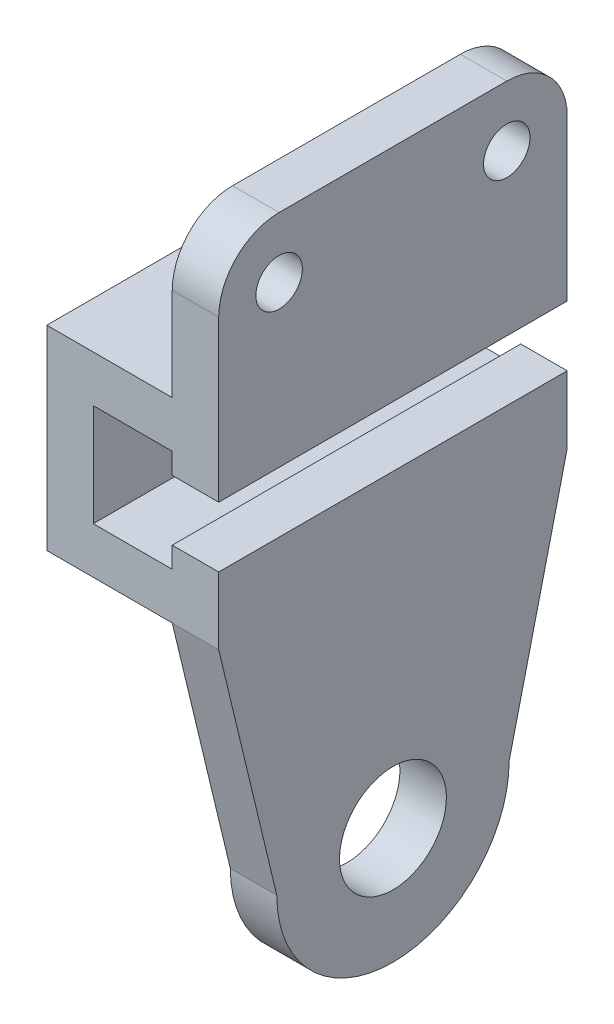
ISO-10303-21;
HEADER;
FILE_DESCRIPTION(('STEP AP214'),'2;1');
FILE_NAME('part.step','',(''),(''),'','','');
FILE_SCHEMA(('AUTOMOTIVE_DESIGN { 1 0 10303 214 1 1 1 1 }'));
ENDSEC;
DATA;
#1=APPLICATION_CONTEXT('core data for automotive mechanical design processes');
#2=APPLICATION_PROTOCOL_DEFINITION('international standard','automotive_design',2000,#1);
#3=PRODUCT_CONTEXT('',#1,'mechanical');
#4=PRODUCT('Part','Part','',(#3));
#5=PRODUCT_RELATED_PRODUCT_CATEGORY('part','',(#4));
#6=PRODUCT_DEFINITION_FORMATION('','',#4);
#7=PRODUCT_DEFINITION_CONTEXT('part definition',#1,'design');
#8=PRODUCT_DEFINITION('design','',#6,#7);
#9=PRODUCT_DEFINITION_SHAPE('','',#8);
#10=(LENGTH_UNIT() NAMED_UNIT(*) SI_UNIT(.MILLI.,.METRE.));
#11=(NAMED_UNIT(*) PLANE_ANGLE_UNIT() SI_UNIT($,.RADIAN.));
#12=(NAMED_UNIT(*) SI_UNIT($,.STERADIAN.) SOLID_ANGLE_UNIT());
#13=UNCERTAINTY_MEASURE_WITH_UNIT(LENGTH_MEASURE(1.E-05),#10,'distance_accuracy_value','');
#14=(GEOMETRIC_REPRESENTATION_CONTEXT(3) GLOBAL_UNCERTAINTY_ASSIGNED_CONTEXT((#13)) GLOBAL_UNIT_ASSIGNED_CONTEXT((#10,
#11,#12)) REPRESENTATION_CONTEXT('',''));
#15=CARTESIAN_POINT('',(0.,0.,0.));
#16=DIRECTION('',(0.,0.,1.));
#17=DIRECTION('',(1.,0.,0.));
#18=AXIS2_PLACEMENT_3D('',#15,#16,#17);
#19=CARTESIAN_POINT('',(0.,0.,37.5));
#20=DIRECTION('',(0.,0.,1.));
#21=DIRECTION('',(1.,0.,0.));
#22=AXIS2_PLACEMENT_3D('',#19,#20,#21);
#23=PLANE('',#22);
#24=DIRECTION('',(1.,0.,0.));
#25=VECTOR('',#24,1.);
#26=CARTESIAN_POINT('',(-27.,-21.,37.5));
#27=LINE('',#26,#25);
#28=CARTESIAN_POINT('',(-27.,-21.,37.5));
#29=VERTEX_POINT('',#28);
#30=CARTESIAN_POINT('',(0.,-21.,37.5));
#31=VERTEX_POINT('',#30);
#32=EDGE_CURVE('E316',#29,#31,#27,.T.);
#33=ORIENTED_EDGE('',*,*,#32,.T.);
#34=DIRECTION('',(-1.,0.,0.));
#35=VECTOR('',#34,1.);
#36=CARTESIAN_POINT('',(75.,-21.,37.5));
#37=LINE('',#36,#35);
#38=CARTESIAN_POINT('',(9.99999999999999,-21.,37.5));
#39=VERTEX_POINT('',#38);
#40=EDGE_CURVE('E199',#39,#31,#37,.T.);
#41=ORIENTED_EDGE('',*,*,#40,.F.);
#42=DIRECTION('',(0.,1.,0.));
#43=VECTOR('',#42,1.);
#44=CARTESIAN_POINT('',(10.,-21.,37.5));
#45=LINE('',#44,#43);
#46=CARTESIAN_POINT('',(10.,-6.5,37.5));
#47=VERTEX_POINT('',#46);
#48=EDGE_CURVE('E229',#39,#47,#45,.T.);
#49=ORIENTED_EDGE('',*,*,#48,.T.);
#50=DIRECTION('',(-1.,0.,0.));
#51=VECTOR('',#50,1.);
#52=CARTESIAN_POINT('',(0.,-6.5,37.5));
#53=LINE('',#52,#51);
#54=CARTESIAN_POINT('',(0.,-6.5,37.5));
#55=VERTEX_POINT('',#54);
#56=EDGE_CURVE('E245',#47,#55,#53,.T.);
#57=ORIENTED_EDGE('',*,*,#56,.T.);
#58=DIRECTION('',(0.,-1.,0.));
#59=VECTOR('',#58,1.);
#60=CARTESIAN_POINT('',(0.,-21.,37.5));
#61=LINE('',#60,#59);
#62=CARTESIAN_POINT('',(0.,-11.,37.5));
#63=VERTEX_POINT('',#62);
#64=EDGE_CURVE('E231',#55,#63,#61,.T.);
#65=ORIENTED_EDGE('',*,*,#64,.T.);
#66=DIRECTION('',(-1.,0.,0.));
#67=VECTOR('',#66,1.);
#68=CARTESIAN_POINT('',(0.,-11.,37.5));
#69=LINE('',#68,#67);
#70=CARTESIAN_POINT('',(-17.,-11.,37.5));
#71=VERTEX_POINT('',#70);
#72=EDGE_CURVE('E318',#63,#71,#69,.T.);
#73=ORIENTED_EDGE('',*,*,#72,.T.);
#74=DIRECTION('',(0.,1.,0.));
#75=VECTOR('',#74,1.);
#76=CARTESIAN_POINT('',(-17.,-11.,37.5));
#77=LINE('',#76,#75);
#78=CARTESIAN_POINT('',(-17.,11.,37.5));
#79=VERTEX_POINT('',#78);
#80=EDGE_CURVE('E319',#71,#79,#77,.T.);
#81=ORIENTED_EDGE('',*,*,#80,.T.);
#82=DIRECTION('',(1.,0.,0.));
#83=VECTOR('',#82,1.);
#84=CARTESIAN_POINT('',(-17.,11.,37.5));
#85=LINE('',#84,#83);
#86=CARTESIAN_POINT('',(0.,11.,37.5));
#87=VERTEX_POINT('',#86);
#88=EDGE_CURVE('E325',#79,#87,#85,.T.);
#89=ORIENTED_EDGE('',*,*,#88,.T.);
#90=DIRECTION('',(0.,-1.,0.));
#91=VECTOR('',#90,1.);
#92=CARTESIAN_POINT('',(0.,21.,37.5));
#93=LINE('',#92,#91);
#94=CARTESIAN_POINT('',(0.,6.5,37.5));
#95=VERTEX_POINT('',#94);
#96=EDGE_CURVE('E299',#87,#95,#93,.T.);
#97=ORIENTED_EDGE('',*,*,#96,.T.);
#98=DIRECTION('',(1.,0.,0.));
#99=VECTOR('',#98,1.);
#100=CARTESIAN_POINT('',(0.,6.5,37.5));
#101=LINE('',#100,#99);
#102=CARTESIAN_POINT('',(10.,6.5,37.5));
#103=VERTEX_POINT('',#102);
#104=EDGE_CURVE('E286',#95,#103,#101,.T.);
#105=ORIENTED_EDGE('',*,*,#104,.T.);
#106=DIRECTION('',(0.,1.,0.));
#107=VECTOR('',#106,1.);
#108=CARTESIAN_POINT('',(10.,54.,37.5));
#109=LINE('',#108,#107);
#110=CARTESIAN_POINT('',(10.,41.,37.5));
#111=VERTEX_POINT('',#110);
#112=EDGE_CURVE('E291',#103,#111,#109,.T.);
#113=ORIENTED_EDGE('',*,*,#112,.T.);
#114=DIRECTION('',(-1.,0.,0.));
#115=VECTOR('',#114,1.);
#116=CARTESIAN_POINT('',(0.,41.,37.5));
#117=LINE('',#116,#115);
#118=CARTESIAN_POINT('',(0.,41.,37.5));
#119=VERTEX_POINT('',#118);
#120=EDGE_CURVE('E359',#111,#119,#117,.T.);
#121=ORIENTED_EDGE('',*,*,#120,.T.);
#122=CARTESIAN_POINT('',(0.,21.,37.5));
#123=VERTEX_POINT('',#122);
#124=EDGE_CURVE('E300',#119,#123,#93,.T.);
#125=ORIENTED_EDGE('',*,*,#124,.T.);
#126=DIRECTION('',(-1.,0.,0.));
#127=VECTOR('',#126,1.);
#128=CARTESIAN_POINT('',(0.,21.,37.5));
#129=LINE('',#128,#127);
#130=CARTESIAN_POINT('',(-27.,21.,37.5));
#131=VERTEX_POINT('',#130);
#132=EDGE_CURVE('E309',#123,#131,#129,.T.);
#133=ORIENTED_EDGE('',*,*,#132,.T.);
#134=DIRECTION('',(0.,-1.,0.));
#135=VECTOR('',#134,1.);
#136=CARTESIAN_POINT('',(-27.,21.,37.5));
#137=LINE('',#136,#135);
#138=EDGE_CURVE('E311',#131,#29,#137,.T.);
#139=ORIENTED_EDGE('',*,*,#138,.T.);
#140=EDGE_LOOP('',(#33,#41,#49,#57,#65,#73,#81,#89,#97,#105,#113,#121,#125,#133,#139));
#141=FACE_BOUND('',#140,.T.);
#142=ADVANCED_FACE('F44',(#141),#23,.T.);
#143=CARTESIAN_POINT('',(0.,0.,-37.5));
#144=DIRECTION('',(0.,0.,1.));
#145=DIRECTION('',(1.,0.,0.));
#146=AXIS2_PLACEMENT_3D('',#143,#144,#145);
#147=PLANE('',#146);
#148=DIRECTION('',(-1.,0.,0.));
#149=VECTOR('',#148,1.);
#150=CARTESIAN_POINT('',(75.,-21.,-37.5));
#151=LINE('',#150,#149);
#152=CARTESIAN_POINT('',(10.,-21.,-37.5));
#153=VERTEX_POINT('',#152);
#154=CARTESIAN_POINT('',(0.,-21.,-37.5));
#155=VERTEX_POINT('',#154);
#156=EDGE_CURVE('E58',#153,#155,#151,.T.);
#157=ORIENTED_EDGE('',*,*,#156,.T.);
#158=DIRECTION('',(1.,0.,0.));
#159=VECTOR('',#158,1.);
#160=CARTESIAN_POINT('',(-27.,-21.,-37.5));
#161=LINE('',#160,#159);
#162=CARTESIAN_POINT('',(-27.,-21.,-37.5));
#163=VERTEX_POINT('',#162);
#164=EDGE_CURVE('E328',#163,#155,#161,.T.);
#165=ORIENTED_EDGE('',*,*,#164,.F.);
#166=DIRECTION('',(0.,-1.,0.));
#167=VECTOR('',#166,1.);
#168=CARTESIAN_POINT('',(-27.,21.,-37.5));
#169=LINE('',#168,#167);
#170=CARTESIAN_POINT('',(-27.,21.,-37.5));
#171=VERTEX_POINT('',#170);
#172=EDGE_CURVE('E330',#171,#163,#169,.T.);
#173=ORIENTED_EDGE('',*,*,#172,.F.);
#174=DIRECTION('',(-1.,0.,0.));
#175=VECTOR('',#174,1.);
#176=CARTESIAN_POINT('',(0.,21.,-37.5));
#177=LINE('',#176,#175);
#178=CARTESIAN_POINT('',(0.,21.,-37.5));
#179=VERTEX_POINT('',#178);
#180=EDGE_CURVE('E305',#179,#171,#177,.T.);
#181=ORIENTED_EDGE('',*,*,#180,.F.);
#182=DIRECTION('',(0.,-1.,0.));
#183=VECTOR('',#182,1.);
#184=CARTESIAN_POINT('',(0.,21.,-37.5));
#185=LINE('',#184,#183);
#186=CARTESIAN_POINT('',(0.,41.,-37.5));
#187=VERTEX_POINT('',#186);
#188=EDGE_CURVE('E278',#187,#179,#185,.T.);
#189=ORIENTED_EDGE('',*,*,#188,.F.);
#190=DIRECTION('',(-1.,0.,0.));
#191=VECTOR('',#190,1.);
#192=CARTESIAN_POINT('',(10.,41.,-37.5));
#193=LINE('',#192,#191);
#194=CARTESIAN_POINT('',(10.,41.,-37.5));
#195=VERTEX_POINT('',#194);
#196=EDGE_CURVE('E374',#187,#195,#193,.F.);
#197=ORIENTED_EDGE('',*,*,#196,.T.);
#198=DIRECTION('',(0.,1.,0.));
#199=VECTOR('',#198,1.);
#200=CARTESIAN_POINT('',(10.,6.5,-37.5));
#201=LINE('',#200,#199);
#202=CARTESIAN_POINT('',(10.,6.5,-37.5));
#203=VERTEX_POINT('',#202);
#204=EDGE_CURVE('E287',#203,#195,#201,.T.);
#205=ORIENTED_EDGE('',*,*,#204,.F.);
#206=DIRECTION('',(1.,0.,0.));
#207=VECTOR('',#206,1.);
#208=CARTESIAN_POINT('',(0.,6.5,-37.5));
#209=LINE('',#208,#207);
#210=CARTESIAN_POINT('',(0.,6.5,-37.5));
#211=VERTEX_POINT('',#210);
#212=EDGE_CURVE('E284',#211,#203,#209,.T.);
#213=ORIENTED_EDGE('',*,*,#212,.F.);
#214=CARTESIAN_POINT('',(0.,11.,-37.5));
#215=VERTEX_POINT('',#214);
#216=EDGE_CURVE('E285',#215,#211,#185,.T.);
#217=ORIENTED_EDGE('',*,*,#216,.F.);
#218=DIRECTION('',(1.,0.,0.));
#219=VECTOR('',#218,1.);
#220=CARTESIAN_POINT('',(-17.,11.,-37.5));
#221=LINE('',#220,#219);
#222=CARTESIAN_POINT('',(-17.,11.,-37.5));
#223=VERTEX_POINT('',#222);
#224=EDGE_CURVE('E314',#223,#215,#221,.T.);
#225=ORIENTED_EDGE('',*,*,#224,.F.);
#226=DIRECTION('',(0.,1.,0.));
#227=VECTOR('',#226,1.);
#228=CARTESIAN_POINT('',(-17.,-11.,-37.5));
#229=LINE('',#228,#227);
#230=CARTESIAN_POINT('',(-17.,-11.,-37.5));
#231=VERTEX_POINT('',#230);
#232=EDGE_CURVE('E331',#231,#223,#229,.T.);
#233=ORIENTED_EDGE('',*,*,#232,.F.);
#234=DIRECTION('',(-1.,0.,0.));
#235=VECTOR('',#234,1.);
#236=CARTESIAN_POINT('',(0.,-11.,-37.5));
#237=LINE('',#236,#235);
#238=CARTESIAN_POINT('',(0.,-11.,-37.5));
#239=VERTEX_POINT('',#238);
#240=EDGE_CURVE('E335',#239,#231,#237,.T.);
#241=ORIENTED_EDGE('',*,*,#240,.F.);
#242=DIRECTION('',(0.,-1.,0.));
#243=VECTOR('',#242,1.);
#244=CARTESIAN_POINT('',(0.,-6.5,-37.5));
#245=LINE('',#244,#243);
#246=CARTESIAN_POINT('',(0.,-6.5,-37.5));
#247=VERTEX_POINT('',#246);
#248=EDGE_CURVE('E236',#247,#239,#245,.T.);
#249=ORIENTED_EDGE('',*,*,#248,.F.);
#250=DIRECTION('',(-1.,0.,0.));
#251=VECTOR('',#250,1.);
#252=CARTESIAN_POINT('',(0.,-6.5,-37.5));
#253=LINE('',#252,#251);
#254=CARTESIAN_POINT('',(10.,-6.5,-37.5));
#255=VERTEX_POINT('',#254);
#256=EDGE_CURVE('E234',#255,#247,#253,.T.);
#257=ORIENTED_EDGE('',*,*,#256,.F.);
#258=DIRECTION('',(0.,1.,0.));
#259=VECTOR('',#258,1.);
#260=CARTESIAN_POINT('',(10.,-73.,-37.5));
#261=LINE('',#260,#259);
#262=EDGE_CURVE('E235',#153,#255,#261,.T.);
#263=ORIENTED_EDGE('',*,*,#262,.F.);
#264=EDGE_LOOP('',(#157,#165,#173,#181,#189,#197,#205,#213,#217,#225,#233,#241,#249,#257,#263));
#265=FACE_BOUND('',#264,.T.);
#266=ADVANCED_FACE('F396',(#265),#147,.F.);
#267=CARTESIAN_POINT('',(0.,-21.,-37.5));
#268=DIRECTION('',(-1.,0.,0.));
#269=DIRECTION('',(0.,-1.,0.));
#270=AXIS2_PLACEMENT_3D('',#267,#268,#269);
#271=PLANE('',#270);
#272=CARTESIAN_POINT('',(0.,-73.,0.));
#273=DIRECTION('',(-1.,0.,0.));
#274=DIRECTION('',(0.,-1.,0.));
#275=AXIS2_PLACEMENT_3D('',#272,#273,#274);
#276=CIRCLE('',#275,11.5);
#277=CARTESIAN_POINT('',(0.,-84.5,0.));
#278=VERTEX_POINT('',#277);
#279=EDGE_CURVE('E224',#278,#278,#276,.T.);
#280=ORIENTED_EDGE('',*,*,#279,.F.);
#281=EDGE_LOOP('',(#280));
#282=FACE_BOUND('',#281,.T.);
#283=DIRECTION('',(0.,-0.972302374804256,0.233726532404869));
#284=VECTOR('',#283,1.);
#285=CARTESIAN_POINT('',(0.,-9.66917227515077,-40.2237566646272));
#286=LINE('',#285,#284);
#287=CARTESIAN_POINT('',(0.,-73.,-25.));
#288=VERTEX_POINT('',#287);
#289=EDGE_CURVE('E217',#155,#288,#286,.T.);
#290=ORIENTED_EDGE('',*,*,#289,.T.);
#291=CARTESIAN_POINT('',(0.,-73.,0.));
#292=DIRECTION('',(-1.,0.,0.));
#293=DIRECTION('',(0.,-1.,0.));
#294=AXIS2_PLACEMENT_3D('',#291,#292,#293);
#295=CIRCLE('',#294,25.);
#296=CARTESIAN_POINT('',(0.,-73.,25.));
#297=VERTEX_POINT('',#296);
#298=EDGE_CURVE('E215',#288,#297,#295,.T.);
#299=ORIENTED_EDGE('',*,*,#298,.T.);
#300=DIRECTION('',(0.,0.972302374804256,0.233726532404869));
#301=VECTOR('',#300,1.);
#302=CARTESIAN_POINT('',(0.,-9.66917227515077,40.2237566646272));
#303=LINE('',#302,#301);
#304=EDGE_CURVE('E197',#297,#31,#303,.T.);
#305=ORIENTED_EDGE('',*,*,#304,.T.);
#306=DIRECTION('',(0.,0.,-1.));
#307=VECTOR('',#306,1.);
#308=CARTESIAN_POINT('',(0.,-21.,37.5));
#309=LINE('',#308,#307);
#310=EDGE_CURVE('E352',#31,#155,#309,.T.);
#311=ORIENTED_EDGE('',*,*,#310,.T.);
#312=EDGE_LOOP('',(#290,#299,#305,#311));
#313=FACE_BOUND('',#312,.T.);
#314=ADVANCED_FACE('F220',(#282,#313),#271,.T.);
#315=CARTESIAN_POINT('',(10.,-21.,-37.5));
#316=DIRECTION('',(1.,0.,0.));
#317=DIRECTION('',(0.,0.,-1.));
#318=AXIS2_PLACEMENT_3D('',#315,#316,#317);
#319=PLANE('',#318);
#320=CARTESIAN_POINT('',(10.,-73.,0.));
#321=DIRECTION('',(-1.,0.,0.));
#322=DIRECTION('',(0.,-1.,0.));
#323=AXIS2_PLACEMENT_3D('',#320,#321,#322);
#324=CIRCLE('',#323,11.5);
#325=CARTESIAN_POINT('',(10.,-84.5,0.));
#326=VERTEX_POINT('',#325);
#327=EDGE_CURVE('E218',#326,#326,#324,.T.);
#328=ORIENTED_EDGE('',*,*,#327,.T.);
#329=EDGE_LOOP('',(#328));
#330=FACE_BOUND('',#329,.T.);
#331=DIRECTION('',(0.,-0.972302374804256,-0.233726532404869));
#332=VECTOR('',#331,1.);
#333=CARTESIAN_POINT('',(10.,-38.0439646884014,33.4028931037497));
#334=LINE('',#333,#332);
#335=CARTESIAN_POINT('',(10.,-73.,25.));
#336=VERTEX_POINT('',#335);
#337=EDGE_CURVE('E11',#39,#336,#334,.T.);
#338=ORIENTED_EDGE('',*,*,#337,.T.);
#339=CARTESIAN_POINT('',(10.,-73.,0.));
#340=DIRECTION('',(-1.,0.,0.));
#341=DIRECTION('',(0.,-1.,0.));
#342=AXIS2_PLACEMENT_3D('',#339,#340,#341);
#343=CIRCLE('',#342,25.);
#344=CARTESIAN_POINT('',(10.,-73.,-25.));
#345=VERTEX_POINT('',#344);
#346=EDGE_CURVE('E212',#345,#336,#343,.T.);
#347=ORIENTED_EDGE('',*,*,#346,.F.);
#348=DIRECTION('',(0.,0.972302374804256,-0.233726532404869));
#349=VECTOR('',#348,1.);
#350=CARTESIAN_POINT('',(10.,-21.,-37.5));
#351=LINE('',#350,#349);
#352=EDGE_CURVE('E52',#345,#153,#351,.T.);
#353=ORIENTED_EDGE('',*,*,#352,.T.);
#354=ORIENTED_EDGE('',*,*,#262,.T.);
#355=DIRECTION('',(0.,0.,1.));
#356=VECTOR('',#355,1.);
#357=CARTESIAN_POINT('',(10.,-6.5,-37.5));
#358=LINE('',#357,#356);
#359=EDGE_CURVE('E242',#255,#47,#358,.T.);
#360=ORIENTED_EDGE('',*,*,#359,.T.);
#361=ORIENTED_EDGE('',*,*,#48,.F.);
#362=EDGE_LOOP('',(#338,#347,#353,#354,#360,#361));
#363=FACE_BOUND('',#362,.T.);
#364=ADVANCED_FACE('F397',(#330,#363),#319,.T.);
#365=CARTESIAN_POINT('',(0.,21.,37.5));
#366=DIRECTION('',(0.,-1.,0.));
#367=DIRECTION('',(1.,0.,0.));
#368=AXIS2_PLACEMENT_3D('',#365,#366,#367);
#369=PLANE('',#368);
#370=ORIENTED_EDGE('',*,*,#180,.T.);
#371=DIRECTION('',(0.,0.,-1.));
#372=VECTOR('',#371,1.);
#373=CARTESIAN_POINT('',(-27.,21.,37.5));
#374=LINE('',#373,#372);
#375=EDGE_CURVE('E357',#131,#171,#374,.T.);
#376=ORIENTED_EDGE('',*,*,#375,.F.);
#377=ORIENTED_EDGE('',*,*,#132,.F.);
#378=DIRECTION('',(0.,0.,-1.));
#379=VECTOR('',#378,1.);
#380=CARTESIAN_POINT('',(0.,21.,37.5));
#381=LINE('',#380,#379);
#382=EDGE_CURVE('E322',#123,#179,#381,.T.);
#383=ORIENTED_EDGE('',*,*,#382,.T.);
#384=EDGE_LOOP('',(#370,#376,#377,#383));
#385=FACE_BOUND('',#384,.T.);
#386=ADVANCED_FACE('F419',(#385),#369,.F.);
#387=CARTESIAN_POINT('',(-27.,21.,37.5));
#388=DIRECTION('',(1.,0.,0.));
#389=DIRECTION('',(0.,1.,0.));
#390=AXIS2_PLACEMENT_3D('',#387,#388,#389);
#391=PLANE('',#390);
#392=DIRECTION('',(0.,0.,1.));
#393=VECTOR('',#392,1.);
#394=CARTESIAN_POINT('',(-27.,-6.00000000000001,-17.5));
#395=LINE('',#394,#393);
#396=CARTESIAN_POINT('',(-27.,-6.00000000000001,-17.5));
#397=VERTEX_POINT('',#396);
#398=CARTESIAN_POINT('',(-27.,-6.,17.5));
#399=VERTEX_POINT('',#398);
#400=EDGE_CURVE('E254',#397,#399,#395,.T.);
#401=ORIENTED_EDGE('',*,*,#400,.F.);
#402=CARTESIAN_POINT('',(-27.,0.,-17.5));
#403=DIRECTION('',(-1.,0.,0.));
#404=DIRECTION('',(0.,-1.,0.));
#405=AXIS2_PLACEMENT_3D('',#402,#403,#404);
#406=CIRCLE('',#405,6.);
#407=CARTESIAN_POINT('',(-27.,6.,-17.5));
#408=VERTEX_POINT('',#407);
#409=EDGE_CURVE('E253',#408,#397,#406,.T.);
#410=ORIENTED_EDGE('',*,*,#409,.F.);
#411=DIRECTION('',(0.,0.,-1.));
#412=VECTOR('',#411,1.);
#413=CARTESIAN_POINT('',(-27.,6.,-17.5));
#414=LINE('',#413,#412);
#415=CARTESIAN_POINT('',(-27.,6.,17.5));
#416=VERTEX_POINT('',#415);
#417=EDGE_CURVE('E261',#416,#408,#414,.T.);
#418=ORIENTED_EDGE('',*,*,#417,.F.);
#419=CARTESIAN_POINT('',(-27.,0.,17.5));
#420=DIRECTION('',(-1.,0.,0.));
#421=DIRECTION('',(0.,-1.,0.));
#422=AXIS2_PLACEMENT_3D('',#419,#420,#421);
#423=CIRCLE('',#422,6.);
#424=EDGE_CURVE('E256',#399,#416,#423,.T.);
#425=ORIENTED_EDGE('',*,*,#424,.F.);
#426=EDGE_LOOP('',(#401,#410,#418,#425));
#427=FACE_BOUND('',#426,.T.);
#428=ORIENTED_EDGE('',*,*,#172,.T.);
#429=DIRECTION('',(0.,0.,-1.));
#430=VECTOR('',#429,1.);
#431=CARTESIAN_POINT('',(-27.,-21.,37.5));
#432=LINE('',#431,#430);
#433=EDGE_CURVE('E355',#29,#163,#432,.T.);
#434=ORIENTED_EDGE('',*,*,#433,.F.);
#435=ORIENTED_EDGE('',*,*,#138,.F.);
#436=ORIENTED_EDGE('',*,*,#375,.T.);
#437=EDGE_LOOP('',(#428,#434,#435,#436));
#438=FACE_BOUND('',#437,.T.);
#439=ADVANCED_FACE('F417',(#427,#438),#391,.F.);
#440=CARTESIAN_POINT('',(-27.,-21.,37.5));
#441=DIRECTION('',(0.,1.,0.));
#442=DIRECTION('',(0.,0.,1.));
#443=AXIS2_PLACEMENT_3D('',#440,#441,#442);
#444=PLANE('',#443);
#445=ORIENTED_EDGE('',*,*,#164,.T.);
#446=ORIENTED_EDGE('',*,*,#310,.F.);
#447=ORIENTED_EDGE('',*,*,#32,.F.);
#448=ORIENTED_EDGE('',*,*,#433,.T.);
#449=EDGE_LOOP('',(#445,#446,#447,#448));
#450=FACE_BOUND('',#449,.T.);
#451=ADVANCED_FACE('F415',(#450),#444,.F.);
#452=CARTESIAN_POINT('',(0.,-11.,37.5));
#453=DIRECTION('',(0.,-1.,0.));
#454=DIRECTION('',(1.,0.,0.));
#455=AXIS2_PLACEMENT_3D('',#452,#453,#454);
#456=PLANE('',#455);
#457=ORIENTED_EDGE('',*,*,#240,.T.);
#458=DIRECTION('',(0.,0.,-1.));
#459=VECTOR('',#458,1.);
#460=CARTESIAN_POINT('',(-17.,-11.,37.5));
#461=LINE('',#460,#459);
#462=EDGE_CURVE('E341',#71,#231,#461,.T.);
#463=ORIENTED_EDGE('',*,*,#462,.F.);
#464=ORIENTED_EDGE('',*,*,#72,.F.);
#465=DIRECTION('',(0.,0.,-1.));
#466=VECTOR('',#465,1.);
#467=CARTESIAN_POINT('',(0.,-11.,37.5));
#468=LINE('',#467,#466);
#469=EDGE_CURVE('E346',#63,#239,#468,.T.);
#470=ORIENTED_EDGE('',*,*,#469,.T.);
#471=EDGE_LOOP('',(#457,#463,#464,#470));
#472=FACE_BOUND('',#471,.T.);
#473=ADVANCED_FACE('F465',(#472),#456,.F.);
#474=CARTESIAN_POINT('',(-17.,-11.,37.5));
#475=DIRECTION('',(-1.,0.,0.));
#476=DIRECTION('',(0.,0.,1.));
#477=AXIS2_PLACEMENT_3D('',#474,#475,#476);
#478=PLANE('',#477);
#479=DIRECTION('',(0.,0.,-1.));
#480=VECTOR('',#479,1.);
#481=CARTESIAN_POINT('',(-17.,5.99999999999999,37.5));
#482=LINE('',#481,#480);
#483=CARTESIAN_POINT('',(-17.,6.,17.5));
#484=VERTEX_POINT('',#483);
#485=CARTESIAN_POINT('',(-17.,6.,-17.5));
#486=VERTEX_POINT('',#485);
#487=EDGE_CURVE('E386',#484,#486,#482,.T.);
#488=ORIENTED_EDGE('',*,*,#487,.T.);
#489=CARTESIAN_POINT('',(-17.,0.,-17.5));
#490=DIRECTION('',(-1.,0.,0.));
#491=DIRECTION('',(0.,0.,1.));
#492=AXIS2_PLACEMENT_3D('',#489,#490,#491);
#493=CIRCLE('',#492,6.);
#494=CARTESIAN_POINT('',(-17.,-6.,-17.5));
#495=VERTEX_POINT('',#494);
#496=EDGE_CURVE('E394',#486,#495,#493,.T.);
#497=ORIENTED_EDGE('',*,*,#496,.T.);
#498=DIRECTION('',(0.,0.,1.));
#499=VECTOR('',#498,1.);
#500=CARTESIAN_POINT('',(-17.,-6.,37.5));
#501=LINE('',#500,#499);
#502=CARTESIAN_POINT('',(-17.,-6.,17.5));
#503=VERTEX_POINT('',#502);
#504=EDGE_CURVE('E377',#495,#503,#501,.T.);
#505=ORIENTED_EDGE('',*,*,#504,.T.);
#506=CARTESIAN_POINT('',(-17.,0.,17.5));
#507=DIRECTION('',(-1.,0.,0.));
#508=DIRECTION('',(0.,0.,1.));
#509=AXIS2_PLACEMENT_3D('',#506,#507,#508);
#510=CIRCLE('',#509,6.);
#511=EDGE_CURVE('E387',#503,#484,#510,.T.);
#512=ORIENTED_EDGE('',*,*,#511,.T.);
#513=EDGE_LOOP('',(#488,#497,#505,#512));
#514=FACE_BOUND('',#513,.T.);
#515=ORIENTED_EDGE('',*,*,#232,.T.);
#516=DIRECTION('',(0.,0.,-1.));
#517=VECTOR('',#516,1.);
#518=CARTESIAN_POINT('',(-17.,11.,37.5));
#519=LINE('',#518,#517);
#520=EDGE_CURVE('E345',#79,#223,#519,.T.);
#521=ORIENTED_EDGE('',*,*,#520,.F.);
#522=ORIENTED_EDGE('',*,*,#80,.F.);
#523=ORIENTED_EDGE('',*,*,#462,.T.);
#524=EDGE_LOOP('',(#515,#521,#522,#523));
#525=FACE_BOUND('',#524,.T.);
#526=ADVANCED_FACE('F459',(#514,#525),#478,.F.);
#527=CARTESIAN_POINT('',(-17.,11.,37.5));
#528=DIRECTION('',(0.,1.,0.));
#529=DIRECTION('',(-1.,0.,0.));
#530=AXIS2_PLACEMENT_3D('',#527,#528,#529);
#531=PLANE('',#530);
#532=ORIENTED_EDGE('',*,*,#224,.T.);
#533=DIRECTION('',(0.,0.,-1.));
#534=VECTOR('',#533,1.);
#535=CARTESIAN_POINT('',(0.,11.,37.5));
#536=LINE('',#535,#534);
#537=EDGE_CURVE('E336',#87,#215,#536,.T.);
#538=ORIENTED_EDGE('',*,*,#537,.F.);
#539=ORIENTED_EDGE('',*,*,#88,.F.);
#540=ORIENTED_EDGE('',*,*,#520,.T.);
#541=EDGE_LOOP('',(#532,#538,#539,#540));
#542=FACE_BOUND('',#541,.T.);
#543=ADVANCED_FACE('F451',(#542),#531,.F.);
#544=CARTESIAN_POINT('',(0.,21.,-37.5));
#545=DIRECTION('',(-1.,0.,0.));
#546=DIRECTION('',(0.,0.,1.));
#547=AXIS2_PLACEMENT_3D('',#544,#545,#546);
#548=PLANE('',#547);
#549=CARTESIAN_POINT('',(0.,41.,24.5));
#550=DIRECTION('',(-1.,0.,0.));
#551=DIRECTION('',(0.,0.,1.));
#552=AXIS2_PLACEMENT_3D('',#549,#550,#551);
#553=CIRCLE('',#552,5.);
#554=CARTESIAN_POINT('',(0.,41.,29.5));
#555=VERTEX_POINT('',#554);
#556=EDGE_CURVE('E273',#555,#555,#553,.T.);
#557=ORIENTED_EDGE('',*,*,#556,.F.);
#558=EDGE_LOOP('',(#557));
#559=FACE_BOUND('',#558,.T.);
#560=CARTESIAN_POINT('',(0.,41.,-24.5));
#561=DIRECTION('',(-1.,0.,0.));
#562=DIRECTION('',(0.,0.,1.));
#563=AXIS2_PLACEMENT_3D('',#560,#561,#562);
#564=CIRCLE('',#563,5.);
#565=CARTESIAN_POINT('',(0.,41.,-19.5));
#566=VERTEX_POINT('',#565);
#567=EDGE_CURVE('E270',#566,#566,#564,.T.);
#568=ORIENTED_EDGE('',*,*,#567,.F.);
#569=EDGE_LOOP('',(#568));
#570=FACE_BOUND('',#569,.T.);
#571=DIRECTION('',(0.,0.,1.));
#572=VECTOR('',#571,1.);
#573=CARTESIAN_POINT('',(0.,54.,-37.5));
#574=LINE('',#573,#572);
#575=CARTESIAN_POINT('',(0.,54.,-24.5));
#576=VERTEX_POINT('',#575);
#577=CARTESIAN_POINT('',(0.,54.,24.5));
#578=VERTEX_POINT('',#577);
#579=EDGE_CURVE('E298',#576,#578,#574,.T.);
#580=ORIENTED_EDGE('',*,*,#579,.F.);
#581=CARTESIAN_POINT('',(0.,41.,-24.5));
#582=DIRECTION('',(-1.,0.,0.));
#583=DIRECTION('',(0.,0.,1.));
#584=AXIS2_PLACEMENT_3D('',#581,#582,#583);
#585=CIRCLE('',#584,13.);
#586=EDGE_CURVE('E373',#576,#187,#585,.T.);
#587=ORIENTED_EDGE('',*,*,#586,.T.);
#588=ORIENTED_EDGE('',*,*,#188,.T.);
#589=ORIENTED_EDGE('',*,*,#382,.F.);
#590=ORIENTED_EDGE('',*,*,#124,.F.);
#591=CARTESIAN_POINT('',(0.,41.,24.5));
#592=DIRECTION('',(-1.,0.,0.));
#593=DIRECTION('',(0.,0.,1.));
#594=AXIS2_PLACEMENT_3D('',#591,#592,#593);
#595=CIRCLE('',#594,13.);
#596=EDGE_CURVE('E362',#119,#578,#595,.T.);
#597=ORIENTED_EDGE('',*,*,#596,.T.);
#598=EDGE_LOOP('',(#580,#587,#588,#589,#590,#597));
#599=FACE_BOUND('',#598,.T.);
#600=ADVANCED_FACE('F422',(#559,#570,#599),#548,.T.);
#601=ORIENTED_EDGE('',*,*,#537,.T.);
#602=ORIENTED_EDGE('',*,*,#216,.T.);
#603=DIRECTION('',(0.,0.,1.));
#604=VECTOR('',#603,1.);
#605=CARTESIAN_POINT('',(0.,6.5,-37.5));
#606=LINE('',#605,#604);
#607=EDGE_CURVE('E289',#211,#95,#606,.T.);
#608=ORIENTED_EDGE('',*,*,#607,.T.);
#609=ORIENTED_EDGE('',*,*,#96,.F.);
#610=EDGE_LOOP('',(#601,#602,#608,#609));
#611=FACE_BOUND('',#610,.T.);
#612=ADVANCED_FACE('F452',(#611),#548,.T.);
#613=CARTESIAN_POINT('',(0.,54.,-37.5));
#614=DIRECTION('',(0.,1.,0.));
#615=DIRECTION('',(0.,0.,1.));
#616=AXIS2_PLACEMENT_3D('',#613,#614,#615);
#617=PLANE('',#616);
#618=DIRECTION('',(0.,0.,1.));
#619=VECTOR('',#618,1.);
#620=CARTESIAN_POINT('',(10.,54.,-37.5));
#621=LINE('',#620,#619);
#622=CARTESIAN_POINT('',(10.,54.,-24.5));
#623=VERTEX_POINT('',#622);
#624=CARTESIAN_POINT('',(10.,54.,24.5));
#625=VERTEX_POINT('',#624);
#626=EDGE_CURVE('E303',#623,#625,#621,.T.);
#627=ORIENTED_EDGE('',*,*,#626,.F.);
#628=DIRECTION('',(-1.,0.,0.));
#629=VECTOR('',#628,1.);
#630=CARTESIAN_POINT('',(0.,54.,-24.5));
#631=LINE('',#630,#629);
#632=EDGE_CURVE('E367',#623,#576,#631,.T.);
#633=ORIENTED_EDGE('',*,*,#632,.T.);
#634=ORIENTED_EDGE('',*,*,#579,.T.);
#635=DIRECTION('',(-1.,0.,0.));
#636=VECTOR('',#635,1.);
#637=CARTESIAN_POINT('',(0.,54.,24.5));
#638=LINE('',#637,#636);
#639=EDGE_CURVE('E364',#578,#625,#638,.F.);
#640=ORIENTED_EDGE('',*,*,#639,.T.);
#641=EDGE_LOOP('',(#627,#633,#634,#640));
#642=FACE_BOUND('',#641,.T.);
#643=ADVANCED_FACE('F434',(#642),#617,.T.);
#644=CARTESIAN_POINT('',(10.,54.,-37.5));
#645=DIRECTION('',(1.,0.,0.));
#646=DIRECTION('',(0.,0.,-1.));
#647=AXIS2_PLACEMENT_3D('',#644,#645,#646);
#648=PLANE('',#647);
#649=CARTESIAN_POINT('',(9.99999999999999,41.,24.5));
#650=DIRECTION('',(1.,0.,0.));
#651=DIRECTION('',(0.,0.,-1.));
#652=AXIS2_PLACEMENT_3D('',#649,#650,#651);
#653=CIRCLE('',#652,5.);
#654=CARTESIAN_POINT('',(9.99999999999999,41.,19.5));
#655=VERTEX_POINT('',#654);
#656=EDGE_CURVE('E294',#655,#655,#653,.T.);
#657=ORIENTED_EDGE('',*,*,#656,.F.);
#658=EDGE_LOOP('',(#657));
#659=FACE_BOUND('',#658,.T.);
#660=CARTESIAN_POINT('',(9.99999999999999,41.,-24.5));
#661=DIRECTION('',(1.,0.,0.));
#662=DIRECTION('',(0.,0.,-1.));
#663=AXIS2_PLACEMENT_3D('',#660,#661,#662);
#664=CIRCLE('',#663,5.);
#665=CARTESIAN_POINT('',(9.99999999999999,41.,-29.5));
#666=VERTEX_POINT('',#665);
#667=EDGE_CURVE('E280',#666,#666,#664,.T.);
#668=ORIENTED_EDGE('',*,*,#667,.F.);
#669=EDGE_LOOP('',(#668));
#670=FACE_BOUND('',#669,.T.);
#671=ORIENTED_EDGE('',*,*,#204,.T.);
#672=CARTESIAN_POINT('',(10.,41.,-24.5));
#673=DIRECTION('',(1.,0.,0.));
#674=DIRECTION('',(0.,0.,-1.));
#675=AXIS2_PLACEMENT_3D('',#672,#673,#674);
#676=CIRCLE('',#675,13.);
#677=EDGE_CURVE('E380',#195,#623,#676,.T.);
#678=ORIENTED_EDGE('',*,*,#677,.T.);
#679=ORIENTED_EDGE('',*,*,#626,.T.);
#680=CARTESIAN_POINT('',(10.,41.,24.5));
#681=DIRECTION('',(1.,0.,0.));
#682=DIRECTION('',(0.,0.,-1.));
#683=AXIS2_PLACEMENT_3D('',#680,#681,#682);
#684=CIRCLE('',#683,13.);
#685=EDGE_CURVE('E366',#625,#111,#684,.T.);
#686=ORIENTED_EDGE('',*,*,#685,.T.);
#687=ORIENTED_EDGE('',*,*,#112,.F.);
#688=DIRECTION('',(0.,0.,1.));
#689=VECTOR('',#688,1.);
#690=CARTESIAN_POINT('',(10.,6.5,-37.5));
#691=LINE('',#690,#689);
#692=EDGE_CURVE('E301',#203,#103,#691,.T.);
#693=ORIENTED_EDGE('',*,*,#692,.F.);
#694=EDGE_LOOP('',(#671,#678,#679,#686,#687,#693));
#695=FACE_BOUND('',#694,.T.);
#696=ADVANCED_FACE('F433',(#659,#670,#695),#648,.T.);
#697=CARTESIAN_POINT('',(0.,6.5,-37.5));
#698=DIRECTION('',(0.,-1.,0.));
#699=DIRECTION('',(0.,0.,-1.));
#700=AXIS2_PLACEMENT_3D('',#697,#698,#699);
#701=PLANE('',#700);
#702=ORIENTED_EDGE('',*,*,#104,.F.);
#703=ORIENTED_EDGE('',*,*,#607,.F.);
#704=ORIENTED_EDGE('',*,*,#212,.T.);
#705=ORIENTED_EDGE('',*,*,#692,.T.);
#706=EDGE_LOOP('',(#702,#703,#704,#705));
#707=FACE_BOUND('',#706,.T.);
#708=ADVANCED_FACE('F443',(#707),#701,.T.);
#709=CARTESIAN_POINT('',(0.,41.,24.5));
#710=DIRECTION('',(-1.,0.,0.));
#711=DIRECTION('',(0.,0.,1.));
#712=AXIS2_PLACEMENT_3D('',#709,#710,#711);
#713=CYLINDRICAL_SURFACE('',#712,13.);
#714=ORIENTED_EDGE('',*,*,#685,.F.);
#715=ORIENTED_EDGE('',*,*,#639,.F.);
#716=ORIENTED_EDGE('',*,*,#596,.F.);
#717=ORIENTED_EDGE('',*,*,#120,.F.);
#718=EDGE_LOOP('',(#714,#715,#716,#717));
#719=FACE_BOUND('',#718,.T.);
#720=ADVANCED_FACE('F439',(#719),#713,.T.);
#721=CARTESIAN_POINT('',(0.,41.,-24.5));
#722=DIRECTION('',(1.,0.,0.));
#723=DIRECTION('',(0.,0.,-1.));
#724=AXIS2_PLACEMENT_3D('',#721,#722,#723);
#725=CYLINDRICAL_SURFACE('',#724,13.);
#726=ORIENTED_EDGE('',*,*,#677,.F.);
#727=ORIENTED_EDGE('',*,*,#196,.F.);
#728=ORIENTED_EDGE('',*,*,#586,.F.);
#729=ORIENTED_EDGE('',*,*,#632,.F.);
#730=EDGE_LOOP('',(#726,#727,#728,#729));
#731=FACE_BOUND('',#730,.T.);
#732=ADVANCED_FACE('F50',(#731),#725,.T.);
#733=CARTESIAN_POINT('',(75.,41.,-24.5));
#734=DIRECTION('',(-1.,0.,0.));
#735=DIRECTION('',(0.,0.,1.));
#736=AXIS2_PLACEMENT_3D('',#733,#734,#735);
#737=CYLINDRICAL_SURFACE('',#736,5.);
#738=ORIENTED_EDGE('',*,*,#667,.T.);
#739=EDGE_LOOP('',(#738));
#740=FACE_BOUND('',#739,.T.);
#741=ORIENTED_EDGE('',*,*,#567,.T.);
#742=EDGE_LOOP('',(#741));
#743=FACE_BOUND('',#742,.T.);
#744=ADVANCED_FACE('F509',(#740,#743),#737,.F.);
#745=CARTESIAN_POINT('',(75.,41.,24.5));
#746=DIRECTION('',(-1.,0.,0.));
#747=DIRECTION('',(0.,0.,1.));
#748=AXIS2_PLACEMENT_3D('',#745,#746,#747);
#749=CYLINDRICAL_SURFACE('',#748,5.);
#750=ORIENTED_EDGE('',*,*,#656,.T.);
#751=EDGE_LOOP('',(#750));
#752=FACE_BOUND('',#751,.T.);
#753=ORIENTED_EDGE('',*,*,#556,.T.);
#754=EDGE_LOOP('',(#753));
#755=FACE_BOUND('',#754,.T.);
#756=ADVANCED_FACE('F527',(#752,#755),#749,.F.);
#757=CARTESIAN_POINT('',(48.,0.,-17.5));
#758=DIRECTION('',(-1.,0.,0.));
#759=DIRECTION('',(0.,-1.,0.));
#760=AXIS2_PLACEMENT_3D('',#757,#758,#759);
#761=CYLINDRICAL_SURFACE('',#760,6.);
#762=DIRECTION('',(-1.,0.,0.));
#763=VECTOR('',#762,1.);
#764=CARTESIAN_POINT('',(48.,6.,-17.5));
#765=LINE('',#764,#763);
#766=EDGE_CURVE('E264',#486,#408,#765,.T.);
#767=ORIENTED_EDGE('',*,*,#766,.T.);
#768=ORIENTED_EDGE('',*,*,#409,.T.);
#769=DIRECTION('',(-1.,0.,0.));
#770=VECTOR('',#769,1.);
#771=CARTESIAN_POINT('',(48.,-6.,-17.5));
#772=LINE('',#771,#770);
#773=EDGE_CURVE('E262',#495,#397,#772,.T.);
#774=ORIENTED_EDGE('',*,*,#773,.F.);
#775=ORIENTED_EDGE('',*,*,#496,.F.);
#776=EDGE_LOOP('',(#767,#768,#774,#775));
#777=FACE_BOUND('',#776,.T.);
#778=ADVANCED_FACE('F533',(#777),#761,.F.);
#779=CARTESIAN_POINT('',(48.,6.,-17.5));
#780=DIRECTION('',(0.,1.,0.));
#781=DIRECTION('',(-1.,0.,0.));
#782=AXIS2_PLACEMENT_3D('',#779,#780,#781);
#783=PLANE('',#782);
#784=DIRECTION('',(-1.,0.,0.));
#785=VECTOR('',#784,1.);
#786=CARTESIAN_POINT('',(48.,6.,17.5));
#787=LINE('',#786,#785);
#788=EDGE_CURVE('E268',#484,#416,#787,.T.);
#789=ORIENTED_EDGE('',*,*,#788,.T.);
#790=ORIENTED_EDGE('',*,*,#417,.T.);
#791=ORIENTED_EDGE('',*,*,#766,.F.);
#792=ORIENTED_EDGE('',*,*,#487,.F.);
#793=EDGE_LOOP('',(#789,#790,#791,#792));
#794=FACE_BOUND('',#793,.T.);
#795=ADVANCED_FACE('F534',(#794),#783,.F.);
#796=CARTESIAN_POINT('',(48.,0.,17.5));
#797=DIRECTION('',(-1.,0.,0.));
#798=DIRECTION('',(0.,-1.,0.));
#799=AXIS2_PLACEMENT_3D('',#796,#797,#798);
#800=CYLINDRICAL_SURFACE('',#799,6.);
#801=DIRECTION('',(-1.,0.,0.));
#802=VECTOR('',#801,1.);
#803=CARTESIAN_POINT('',(48.,-5.99999999999999,17.5));
#804=LINE('',#803,#802);
#805=EDGE_CURVE('E269',#503,#399,#804,.T.);
#806=ORIENTED_EDGE('',*,*,#805,.T.);
#807=ORIENTED_EDGE('',*,*,#424,.T.);
#808=ORIENTED_EDGE('',*,*,#788,.F.);
#809=ORIENTED_EDGE('',*,*,#511,.F.);
#810=EDGE_LOOP('',(#806,#807,#808,#809));
#811=FACE_BOUND('',#810,.T.);
#812=ADVANCED_FACE('F478',(#811),#800,.F.);
#813=CARTESIAN_POINT('',(48.,-6.,-17.5));
#814=DIRECTION('',(0.,-1.,0.));
#815=DIRECTION('',(0.,0.,-1.));
#816=AXIS2_PLACEMENT_3D('',#813,#814,#815);
#817=PLANE('',#816);
#818=ORIENTED_EDGE('',*,*,#773,.T.);
#819=ORIENTED_EDGE('',*,*,#400,.T.);
#820=ORIENTED_EDGE('',*,*,#805,.F.);
#821=ORIENTED_EDGE('',*,*,#504,.F.);
#822=EDGE_LOOP('',(#818,#819,#820,#821));
#823=FACE_BOUND('',#822,.T.);
#824=ADVANCED_FACE('F470',(#823),#817,.F.);
#825=ORIENTED_EDGE('',*,*,#469,.F.);
#826=ORIENTED_EDGE('',*,*,#64,.F.);
#827=DIRECTION('',(0.,0.,1.));
#828=VECTOR('',#827,1.);
#829=CARTESIAN_POINT('',(0.,-6.5,-37.5));
#830=LINE('',#829,#828);
#831=EDGE_CURVE('E248',#247,#55,#830,.T.);
#832=ORIENTED_EDGE('',*,*,#831,.F.);
#833=ORIENTED_EDGE('',*,*,#248,.T.);
#834=EDGE_LOOP('',(#825,#826,#832,#833));
#835=FACE_BOUND('',#834,.T.);
#836=ADVANCED_FACE('F463',(#835),#271,.T.);
#837=CARTESIAN_POINT('',(0.,-6.5,-37.5));
#838=DIRECTION('',(0.,1.,0.));
#839=DIRECTION('',(0.,0.,1.));
#840=AXIS2_PLACEMENT_3D('',#837,#838,#839);
#841=PLANE('',#840);
#842=ORIENTED_EDGE('',*,*,#56,.F.);
#843=ORIENTED_EDGE('',*,*,#359,.F.);
#844=ORIENTED_EDGE('',*,*,#256,.T.);
#845=ORIENTED_EDGE('',*,*,#831,.T.);
#846=EDGE_LOOP('',(#842,#843,#844,#845));
#847=FACE_BOUND('',#846,.T.);
#848=ADVANCED_FACE('F403',(#847),#841,.T.);
#849=CARTESIAN_POINT('',(75.,-9.66917227515076,-40.2237566646272));
#850=DIRECTION('',(0.,-0.233726532404869,-0.972302374804256));
#851=DIRECTION('',(0.,0.972302374804256,-0.233726532404869));
#852=AXIS2_PLACEMENT_3D('',#849,#850,#851);
#853=PLANE('',#852);
#854=DIRECTION('',(-1.,0.,0.));
#855=VECTOR('',#854,1.);
#856=CARTESIAN_POINT('',(75.,-73.,-25.));
#857=LINE('',#856,#855);
#858=EDGE_CURVE('E202',#345,#288,#857,.T.);
#859=ORIENTED_EDGE('',*,*,#858,.T.);
#860=ORIENTED_EDGE('',*,*,#289,.F.);
#861=ORIENTED_EDGE('',*,*,#156,.F.);
#862=ORIENTED_EDGE('',*,*,#352,.F.);
#863=EDGE_LOOP('',(#859,#860,#861,#862));
#864=FACE_BOUND('',#863,.T.);
#865=ADVANCED_FACE('F471',(#864),#853,.T.);
#866=CARTESIAN_POINT('',(75.,-9.66917227515076,40.2237566646272));
#867=DIRECTION('',(0.,-0.233726532404869,0.972302374804256));
#868=DIRECTION('',(0.,-0.972302374804256,-0.233726532404869));
#869=AXIS2_PLACEMENT_3D('',#866,#867,#868);
#870=PLANE('',#869);
#871=ORIENTED_EDGE('',*,*,#40,.T.);
#872=ORIENTED_EDGE('',*,*,#304,.F.);
#873=DIRECTION('',(-1.,0.,0.));
#874=VECTOR('',#873,1.);
#875=CARTESIAN_POINT('',(75.,-73.,25.));
#876=LINE('',#875,#874);
#877=EDGE_CURVE('E68',#336,#297,#876,.T.);
#878=ORIENTED_EDGE('',*,*,#877,.F.);
#879=ORIENTED_EDGE('',*,*,#337,.F.);
#880=EDGE_LOOP('',(#871,#872,#878,#879));
#881=FACE_BOUND('',#880,.T.);
#882=ADVANCED_FACE('F196',(#881),#870,.T.);
#883=CARTESIAN_POINT('',(10.,-73.,0.));
#884=DIRECTION('',(-1.,0.,0.));
#885=DIRECTION('',(0.,-1.,0.));
#886=AXIS2_PLACEMENT_3D('',#883,#884,#885);
#887=CYLINDRICAL_SURFACE('',#886,25.);
#888=ORIENTED_EDGE('',*,*,#298,.F.);
#889=ORIENTED_EDGE('',*,*,#858,.F.);
#890=ORIENTED_EDGE('',*,*,#346,.T.);
#891=ORIENTED_EDGE('',*,*,#877,.T.);
#892=EDGE_LOOP('',(#888,#889,#890,#891));
#893=FACE_BOUND('',#892,.T.);
#894=ADVANCED_FACE('F209',(#893),#887,.T.);
#895=CARTESIAN_POINT('',(10.,-73.,0.));
#896=DIRECTION('',(-1.,0.,0.));
#897=DIRECTION('',(0.,-1.,0.));
#898=AXIS2_PLACEMENT_3D('',#895,#896,#897);
#899=CYLINDRICAL_SURFACE('',#898,11.5);
#900=ORIENTED_EDGE('',*,*,#327,.F.);
#901=EDGE_LOOP('',(#900));
#902=FACE_BOUND('',#901,.T.);
#903=ORIENTED_EDGE('',*,*,#279,.T.);
#904=EDGE_LOOP('',(#903));
#905=FACE_BOUND('',#904,.T.);
#906=ADVANCED_FACE('F549',(#902,#905),#899,.F.);
#907=CLOSED_SHELL('',(#142,#266,#314,#364,#386,#439,#451,#473,#526,#543,#600,#612,#643,#696,
#708,#720,#732,#744,#756,#778,#795,#812,#824,#836,#848,#865,#882,#894,#906));
#908=MANIFOLD_SOLID_BREP('B2',#907);
#909=ADVANCED_BREP_SHAPE_REPRESENTATION('',(#18,#908),#14);
#910=SHAPE_DEFINITION_REPRESENTATION(#9,#909);
ENDSEC;
END-ISO-10303-21;
